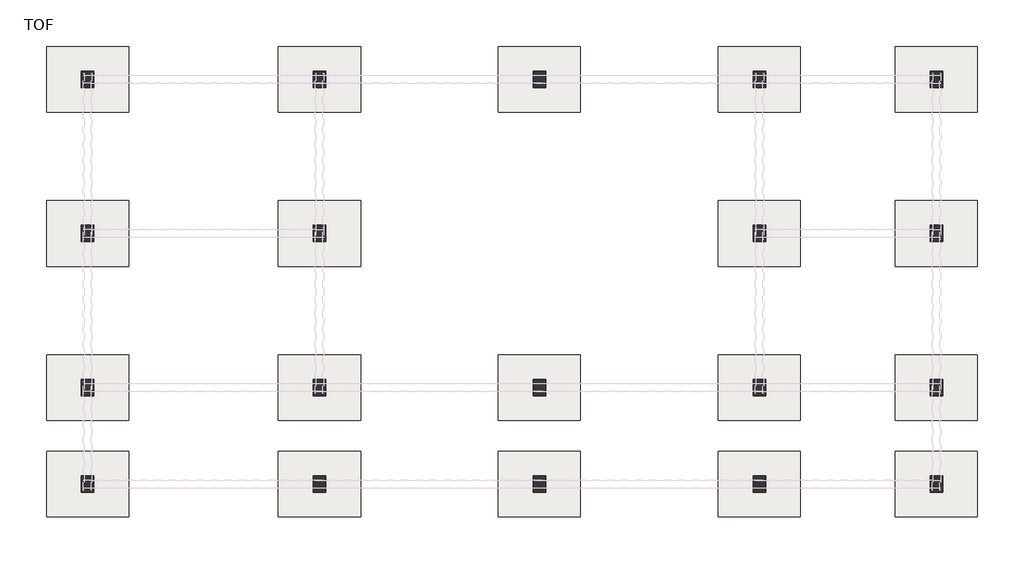
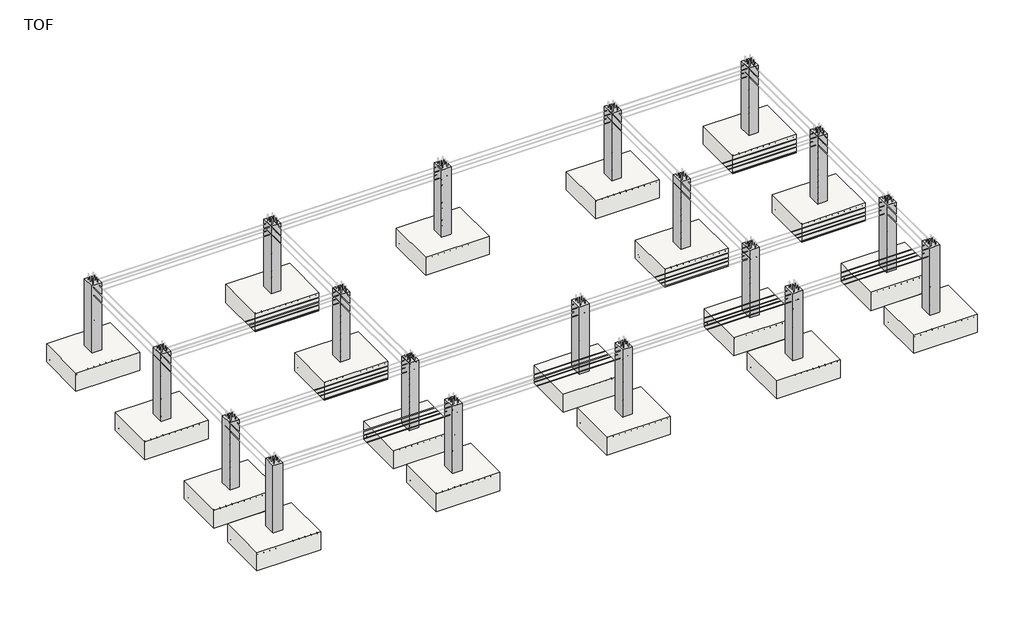
# One storey, part 1 of 10: 19 columns, 19 slabs.
"""IFC4 building model written with IfcOpenShell, lengths in millimetres."""

from ifc_helpers import new_model, si_unit, frame, origin, place, context, project, spatial, polyline, outline, extrude, transform, mapped, element, save
from components import m_footing_rectangular_1500_x_1200_x_450mm_2_af0c1bbe

model = new_model("IFC4")

# Units and contexts
model_context = context("Model", 3, world=origin())
ifc_project = project(units=[si_unit("LENGTHUNIT", "METRE", prefix="MILLI")], contexts=[model_context])

# Site, building, storey
site = spatial("IfcSite", under=ifc_project)
building = spatial("IfcBuilding", under=site)
storey = spatial("IfcBuildingStorey", under=building, Name="TOF", Elevation=-1828.8)

# Columns
placement = place(None, origin())
element("IfcColumn", 1, ObjectType="M_Concrete-Rectangular-Column : 230 x 300mm 2", at=placement, inside=storey, context=model_context, shape_type="SweptSolid", body=[
    extrude(outline(polyline([(-2504.7217857, -14944.6267376), (-2504.7217857, -15244.6267376), (-2734.7217857, -15244.6267376), (-2734.7217857, -14944.6267376), (-2504.7217857, -14944.6267376)])), frame((0.0, 0.0, -1828.8), z_axis=(0.0, 0.0, 1.0), x_axis=(1.0, 0.0, 0.0)), (0.0, 0.0, 1.0), 1678.8),
])
element("IfcColumn", 2, ObjectType="M_Concrete-Rectangular-Column : 230 x 300mm 2", at=placement, inside=storey, context=model_context, shape_type="SweptSolid", body=[
    extrude(outline(polyline([(1725.2782143, -14944.6267376), (1725.2782143, -15244.6267376), (1495.2782143, -15244.6267376), (1495.2782143, -14944.6267376), (1725.2782143, -14944.6267376)])), frame((0.0, 0.0, -1828.8), z_axis=(0.0, 0.0, 1.0), x_axis=(1.0, 0.0, 0.0)), (0.0, 0.0, 1.0), 1678.8),
])
element("IfcColumn", 3, ObjectType="M_Concrete-Rectangular-Column : 230 x 300mm 2", at=placement, inside=storey, context=model_context, shape_type="SweptSolid", body=[
    extrude(outline(polyline([(5740.2782143, -14944.6267376), (5740.2782143, -15244.6267376), (5510.2782143, -15244.6267376), (5510.2782143, -14944.6267376), (5740.2782143, -14944.6267376)])), frame((0.0, 0.0, -1828.8), z_axis=(0.0, 0.0, 1.0), x_axis=(1.0, 0.0, 0.0)), (0.0, 0.0, 1.0), 1678.8),
])
element("IfcColumn", 4, ObjectType="M_Concrete-Rectangular-Column : 230 x 300mm 2", at=placement, inside=storey, context=model_context, shape_type="SweptSolid", body=[
    extrude(outline(polyline([(9755.2782143, -14944.6267376), (9755.2782143, -15244.6267376), (9525.2782143, -15244.6267376), (9525.2782143, -14944.6267376), (9755.2782143, -14944.6267376)])), frame((0.0, 0.0, -1828.8), z_axis=(0.0, 0.0, 1.0), x_axis=(1.0, 0.0, 0.0)), (0.0, 0.0, 1.0), 1678.8),
])
element("IfcColumn", 5, ObjectType="M_Concrete-Rectangular-Column : 230 x 300mm 2", at=placement, inside=storey, context=model_context, shape_type="SweptSolid", body=[
    extrude(outline(polyline([(12985.2782143, -14944.6267376), (12985.2782143, -15244.6267376), (12755.2782143, -15244.6267376), (12755.2782143, -14944.6267376), (12985.2782143, -14944.6267376)])), frame((0.0, 0.0, -1828.8), z_axis=(0.0, 0.0, 1.0), x_axis=(1.0, 0.0, 0.0)), (0.0, 0.0, 1.0), 1678.8),
])
element("IfcColumn", 6, ObjectType="M_Concrete-Rectangular-Column : 230 x 300mm 2", at=placement, inside=storey, context=model_context, shape_type="SweptSolid", body=[
    extrude(outline(polyline([(-2504.7217857, -13179.6267376), (-2504.7217857, -13479.6267376), (-2734.7217857, -13479.6267376), (-2734.7217857, -13179.6267376), (-2504.7217857, -13179.6267376)])), frame((0.0, 0.0, -1828.8), z_axis=(0.0, 0.0, 1.0), x_axis=(1.0, 0.0, 0.0)), (0.0, 0.0, 1.0), 1678.8),
])
element("IfcColumn", 7, ObjectType="M_Concrete-Rectangular-Column : 230 x 300mm 2", at=placement, inside=storey, context=model_context, shape_type="SweptSolid", body=[
    extrude(outline(polyline([(1725.2782143, -13179.6267376), (1725.2782143, -13479.6267376), (1495.2782143, -13479.6267376), (1495.2782143, -13179.6267376), (1725.2782143, -13179.6267376)])), frame((0.0, 0.0, -1828.8), z_axis=(0.0, 0.0, 1.0), x_axis=(1.0, 0.0, 0.0)), (0.0, 0.0, 1.0), 1678.8),
])
element("IfcColumn", 8, ObjectType="M_Concrete-Rectangular-Column : 230 x 300mm 2", at=placement, inside=storey, context=model_context, shape_type="SweptSolid", body=[
    extrude(outline(polyline([(5740.2782143, -13179.6267376), (5740.2782143, -13479.6267376), (5510.2782143, -13479.6267376), (5510.2782143, -13179.6267376), (5740.2782143, -13179.6267376)])), frame((0.0, 0.0, -1828.8), z_axis=(0.0, 0.0, 1.0), x_axis=(1.0, 0.0, 0.0)), (0.0, 0.0, 1.0), 1678.8),
])
element("IfcColumn", 9, ObjectType="M_Concrete-Rectangular-Column : 230 x 300mm 2", at=placement, inside=storey, context=model_context, shape_type="SweptSolid", body=[
    extrude(outline(polyline([(9755.2782143, -13179.6267376), (9755.2782143, -13479.6267376), (9525.2782143, -13479.6267376), (9525.2782143, -13179.6267376), (9755.2782143, -13179.6267376)])), frame((0.0, 0.0, -1828.8), z_axis=(0.0, 0.0, 1.0), x_axis=(1.0, 0.0, 0.0)), (0.0, 0.0, 1.0), 1678.8),
])
element("IfcColumn", 10, ObjectType="M_Concrete-Rectangular-Column : 230 x 300mm 2", at=placement, inside=storey, context=model_context, shape_type="SweptSolid", body=[
    extrude(outline(polyline([(12985.2782143, -13179.6267376), (12985.2782143, -13479.6267376), (12755.2782143, -13479.6267376), (12755.2782143, -13179.6267376), (12985.2782143, -13179.6267376)])), frame((0.0, 0.0, -1828.8), z_axis=(0.0, 0.0, 1.0), x_axis=(1.0, 0.0, 0.0)), (0.0, 0.0, 1.0), 1678.8),
])
element("IfcColumn", 11, ObjectType="M_Concrete-Rectangular-Column : 230 x 300mm 2", at=placement, inside=storey, context=model_context, shape_type="SweptSolid", body=[
    extrude(outline(polyline([(-2504.7217857, -10364.6267376), (-2504.7217857, -10664.6267376), (-2734.7217857, -10664.6267376), (-2734.7217857, -10364.6267376), (-2504.7217857, -10364.6267376)])), frame((0.0, 0.0, -1828.8), z_axis=(0.0, 0.0, 1.0), x_axis=(1.0, 0.0, 0.0)), (0.0, 0.0, 1.0), 1678.8),
])
element("IfcColumn", 12, ObjectType="M_Concrete-Rectangular-Column : 230 x 300mm 2", at=placement, inside=storey, context=model_context, shape_type="SweptSolid", body=[
    extrude(outline(polyline([(1725.2782143, -10364.6267376), (1725.2782143, -10664.6267376), (1495.2782143, -10664.6267376), (1495.2782143, -10364.6267376), (1725.2782143, -10364.6267376)])), frame((0.0, 0.0, -1828.8), z_axis=(0.0, 0.0, 1.0), x_axis=(1.0, 0.0, 0.0)), (0.0, 0.0, 1.0), 1678.8),
])
element("IfcColumn", 13, ObjectType="M_Concrete-Rectangular-Column : 230 x 300mm 2", at=placement, inside=storey, context=model_context, shape_type="SweptSolid", body=[
    extrude(outline(polyline([(9755.2782143, -10364.6267376), (9755.2782143, -10664.6267376), (9525.2782143, -10664.6267376), (9525.2782143, -10364.6267376), (9755.2782143, -10364.6267376)])), frame((0.0, 0.0, -1828.8), z_axis=(0.0, 0.0, 1.0), x_axis=(1.0, 0.0, 0.0)), (0.0, 0.0, 1.0), 1678.8),
])
element("IfcColumn", 14, ObjectType="M_Concrete-Rectangular-Column : 230 x 300mm 2", at=placement, inside=storey, context=model_context, shape_type="SweptSolid", body=[
    extrude(outline(polyline([(12985.2782143, -10364.6267376), (12985.2782143, -10664.6267376), (12755.2782143, -10664.6267376), (12755.2782143, -10364.6267376), (12985.2782143, -10364.6267376)])), frame((0.0, 0.0, -1828.8), z_axis=(0.0, 0.0, 1.0), x_axis=(1.0, 0.0, 0.0)), (0.0, 0.0, 1.0), 1678.8),
])
element("IfcColumn", 15, ObjectType="M_Concrete-Rectangular-Column : 230 x 300mm 2", at=placement, inside=storey, context=model_context, shape_type="SweptSolid", body=[
    extrude(outline(polyline([(-2504.7217857, -7549.6267376), (-2504.7217857, -7849.6267376), (-2734.7217857, -7849.6267376), (-2734.7217857, -7549.6267376), (-2504.7217857, -7549.6267376)])), frame((0.0, 0.0, -1828.8), z_axis=(0.0, 0.0, 1.0), x_axis=(1.0, 0.0, 0.0)), (0.0, 0.0, 1.0), 1678.8),
])
element("IfcColumn", 16, ObjectType="M_Concrete-Rectangular-Column : 230 x 300mm 2", at=placement, inside=storey, context=model_context, shape_type="SweptSolid", body=[
    extrude(outline(polyline([(1725.2782143, -7549.6267376), (1725.2782143, -7849.6267376), (1495.2782143, -7849.6267376), (1495.2782143, -7549.6267376), (1725.2782143, -7549.6267376)])), frame((0.0, 0.0, -1828.8), z_axis=(0.0, 0.0, 1.0), x_axis=(1.0, 0.0, 0.0)), (0.0, 0.0, 1.0), 1678.8),
])
element("IfcColumn", 17, ObjectType="M_Concrete-Rectangular-Column : 230 x 300mm 2", at=placement, inside=storey, context=model_context, shape_type="SweptSolid", body=[
    extrude(outline(polyline([(5740.2782143, -7549.6267376), (5740.2782143, -7849.6267376), (5510.2782143, -7849.6267376), (5510.2782143, -7549.6267376), (5740.2782143, -7549.6267376)])), frame((0.0, 0.0, -1828.8), z_axis=(0.0, 0.0, 1.0), x_axis=(1.0, 0.0, 0.0)), (0.0, 0.0, 1.0), 1678.8),
])
element("IfcColumn", 18, ObjectType="M_Concrete-Rectangular-Column : 230 x 300mm 2", at=placement, inside=storey, context=model_context, shape_type="SweptSolid", body=[
    extrude(outline(polyline([(9755.2782143, -7549.6267376), (9755.2782143, -7849.6267376), (9525.2782143, -7849.6267376), (9525.2782143, -7549.6267376), (9755.2782143, -7549.6267376)])), frame((0.0, 0.0, -1828.8), z_axis=(0.0, 0.0, 1.0), x_axis=(1.0, 0.0, 0.0)), (0.0, 0.0, 1.0), 1678.8),
])
element("IfcColumn", 19, ObjectType="M_Concrete-Rectangular-Column : 230 x 300mm 2", at=placement, inside=storey, context=model_context, shape_type="SweptSolid", body=[
    extrude(outline(polyline([(12985.2782143, -7549.6267376), (12985.2782143, -7849.6267376), (12755.2782143, -7849.6267376), (12755.2782143, -7549.6267376), (12985.2782143, -7549.6267376)])), frame((0.0, 0.0, -1828.8), z_axis=(0.0, 0.0, 1.0), x_axis=(1.0, 0.0, 0.0)), (0.0, 0.0, 1.0), 1678.8),
])

# Slabs
m_footing_rectangular_1500_x_1200_x_450mm_2_shape = m_footing_rectangular_1500_x_1200_x_450mm_2_af0c1bbe(model_context)
element("IfcSlab", 20, ObjectType="M_Footing-Rectangular : 1500 x 1200 x 450mm 2", at=placement, inside=storey, context=model_context, shape_type="MappedRepresentation", body=[
    mapped(m_footing_rectangular_1500_x_1200_x_450mm_2_shape, transform((-2619.7217857, -15094.6267376, -1828.8), x_axis=(0.0, 1.0, 0.0), y_axis=(-1.0, 0.0, 0.0), z_axis=(0.0, 0.0, 1.0))),
])
element("IfcSlab", 21, ObjectType="M_Footing-Rectangular : 1500 x 1200 x 450mm 2", at=placement, inside=storey, context=model_context, shape_type="MappedRepresentation", body=[
    mapped(m_footing_rectangular_1500_x_1200_x_450mm_2_shape, transform((1610.2782143, -15094.6267376, -1828.8), x_axis=(0.0, 1.0, 0.0), y_axis=(-1.0, 0.0, 0.0), z_axis=(0.0, 0.0, 1.0))),
])
element("IfcSlab", 22, ObjectType="M_Footing-Rectangular : 1500 x 1200 x 450mm 2", at=placement, inside=storey, context=model_context, shape_type="MappedRepresentation", body=[
    mapped(m_footing_rectangular_1500_x_1200_x_450mm_2_shape, transform((5625.2782143, -15094.6267376, -1828.8), x_axis=(0.0, 1.0, 0.0), y_axis=(-1.0, 0.0, 0.0), z_axis=(0.0, 0.0, 1.0))),
])
element("IfcSlab", 23, ObjectType="M_Footing-Rectangular : 1500 x 1200 x 450mm 2", at=placement, inside=storey, context=model_context, shape_type="MappedRepresentation", body=[
    mapped(m_footing_rectangular_1500_x_1200_x_450mm_2_shape, transform((9640.2782143, -15094.6267376, -1828.8), x_axis=(0.0, 1.0, 0.0), y_axis=(-1.0, 0.0, 0.0), z_axis=(0.0, 0.0, 1.0))),
])
element("IfcSlab", 24, ObjectType="M_Footing-Rectangular : 1500 x 1200 x 450mm 2", at=placement, inside=storey, context=model_context, shape_type="MappedRepresentation", body=[
    mapped(m_footing_rectangular_1500_x_1200_x_450mm_2_shape, transform((12870.2782143, -15094.6267376, -1828.8), x_axis=(0.0, 1.0, 0.0), y_axis=(-1.0, 0.0, 0.0), z_axis=(0.0, 0.0, 1.0))),
])
element("IfcSlab", 25, ObjectType="M_Footing-Rectangular : 1500 x 1200 x 450mm 2", at=placement, inside=storey, context=model_context, shape_type="MappedRepresentation", body=[
    mapped(m_footing_rectangular_1500_x_1200_x_450mm_2_shape, transform((-2619.7217857, -13329.6267376, -1828.8), x_axis=(0.0, 1.0, 0.0), y_axis=(-1.0, 0.0, 0.0), z_axis=(0.0, 0.0, 1.0))),
])
element("IfcSlab", 26, ObjectType="M_Footing-Rectangular : 1500 x 1200 x 450mm 2", at=placement, inside=storey, context=model_context, shape_type="MappedRepresentation", body=[
    mapped(m_footing_rectangular_1500_x_1200_x_450mm_2_shape, transform((1610.2782143, -13329.6267376, -1828.8), x_axis=(0.0, 1.0, 0.0), y_axis=(-1.0, 0.0, 0.0), z_axis=(0.0, 0.0, 1.0))),
])
element("IfcSlab", 27, ObjectType="M_Footing-Rectangular : 1500 x 1200 x 450mm 2", at=placement, inside=storey, context=model_context, shape_type="MappedRepresentation", body=[
    mapped(m_footing_rectangular_1500_x_1200_x_450mm_2_shape, transform((5625.2782143, -13329.6267376, -1828.8), x_axis=(0.0, 1.0, 0.0), y_axis=(-1.0, 0.0, 0.0), z_axis=(0.0, 0.0, 1.0))),
])
element("IfcSlab", 28, ObjectType="M_Footing-Rectangular : 1500 x 1200 x 450mm 2", at=placement, inside=storey, context=model_context, shape_type="MappedRepresentation", body=[
    mapped(m_footing_rectangular_1500_x_1200_x_450mm_2_shape, transform((9640.2782143, -13329.6267376, -1828.8), x_axis=(0.0, 1.0, 0.0), y_axis=(-1.0, 0.0, 0.0), z_axis=(0.0, 0.0, 1.0))),
])
element("IfcSlab", 29, ObjectType="M_Footing-Rectangular : 1500 x 1200 x 450mm 2", at=placement, inside=storey, context=model_context, shape_type="MappedRepresentation", body=[
    mapped(m_footing_rectangular_1500_x_1200_x_450mm_2_shape, transform((12870.2782143, -13329.6267376, -1828.8), x_axis=(0.0, 1.0, 0.0), y_axis=(-1.0, 0.0, 0.0), z_axis=(0.0, 0.0, 1.0))),
])
element("IfcSlab", 30, ObjectType="M_Footing-Rectangular : 1500 x 1200 x 450mm 2", at=placement, inside=storey, context=model_context, shape_type="MappedRepresentation", body=[
    mapped(m_footing_rectangular_1500_x_1200_x_450mm_2_shape, transform((-2619.7217857, -10514.6267376, -1828.8), x_axis=(0.0, 1.0, 0.0), y_axis=(-1.0, 0.0, 0.0), z_axis=(0.0, 0.0, 1.0))),
])
element("IfcSlab", 31, ObjectType="M_Footing-Rectangular : 1500 x 1200 x 450mm 2", at=placement, inside=storey, context=model_context, shape_type="MappedRepresentation", body=[
    mapped(m_footing_rectangular_1500_x_1200_x_450mm_2_shape, transform((1610.2782143, -10514.6267376, -1828.8), x_axis=(0.0, 1.0, 0.0), y_axis=(-1.0, 0.0, 0.0), z_axis=(0.0, 0.0, 1.0))),
])
element("IfcSlab", 32, ObjectType="M_Footing-Rectangular : 1500 x 1200 x 450mm 2", at=placement, inside=storey, context=model_context, shape_type="MappedRepresentation", body=[
    mapped(m_footing_rectangular_1500_x_1200_x_450mm_2_shape, transform((9640.2782143, -10514.6267376, -1828.8), x_axis=(0.0, 1.0, 0.0), y_axis=(-1.0, 0.0, 0.0), z_axis=(0.0, 0.0, 1.0))),
])
element("IfcSlab", 33, ObjectType="M_Footing-Rectangular : 1500 x 1200 x 450mm 2", at=placement, inside=storey, context=model_context, shape_type="MappedRepresentation", body=[
    mapped(m_footing_rectangular_1500_x_1200_x_450mm_2_shape, transform((12870.2782143, -10514.6267376, -1828.8), x_axis=(0.0, 1.0, 0.0), y_axis=(-1.0, 0.0, 0.0), z_axis=(0.0, 0.0, 1.0))),
])
element("IfcSlab", 34, ObjectType="M_Footing-Rectangular : 1500 x 1200 x 450mm 2", at=placement, inside=storey, context=model_context, shape_type="MappedRepresentation", body=[
    mapped(m_footing_rectangular_1500_x_1200_x_450mm_2_shape, transform((-2619.7217857, -7699.6267376, -1828.8), x_axis=(0.0, 1.0, 0.0), y_axis=(-1.0, 0.0, 0.0), z_axis=(0.0, 0.0, 1.0))),
])
element("IfcSlab", 35, ObjectType="M_Footing-Rectangular : 1500 x 1200 x 450mm 2", at=placement, inside=storey, context=model_context, shape_type="MappedRepresentation", body=[
    mapped(m_footing_rectangular_1500_x_1200_x_450mm_2_shape, transform((1610.2782143, -7699.6267376, -1828.8), x_axis=(0.0, 1.0, 0.0), y_axis=(-1.0, 0.0, 0.0), z_axis=(0.0, 0.0, 1.0))),
])
element("IfcSlab", 36, ObjectType="M_Footing-Rectangular : 1500 x 1200 x 450mm 2", at=placement, inside=storey, context=model_context, shape_type="MappedRepresentation", body=[
    mapped(m_footing_rectangular_1500_x_1200_x_450mm_2_shape, transform((5625.2782143, -7699.6267376, -1828.8), x_axis=(0.0, 1.0, 0.0), y_axis=(-1.0, 0.0, 0.0), z_axis=(0.0, 0.0, 1.0))),
])
element("IfcSlab", 37, ObjectType="M_Footing-Rectangular : 1500 x 1200 x 450mm 2", at=placement, inside=storey, context=model_context, shape_type="MappedRepresentation", body=[
    mapped(m_footing_rectangular_1500_x_1200_x_450mm_2_shape, transform((9640.2782143, -7699.6267376, -1828.8), x_axis=(0.0, 1.0, 0.0), y_axis=(-1.0, 0.0, 0.0), z_axis=(0.0, 0.0, 1.0))),
])
element("IfcSlab", 38, ObjectType="M_Footing-Rectangular : 1500 x 1200 x 450mm 2", at=placement, inside=storey, context=model_context, shape_type="MappedRepresentation", body=[
    mapped(m_footing_rectangular_1500_x_1200_x_450mm_2_shape, transform((12870.2782143, -7699.6267376, -1828.8), x_axis=(0.0, 1.0, 0.0), y_axis=(-1.0, 0.0, 0.0), z_axis=(0.0, 0.0, 1.0))),
])

save(model, "model.ifc")

# Revit data of these elements
# Grids (mm)
#   "1": line (15899.329, -15094.627) -> (-5005.909, -15094.627)
#   "2": line (15899.329, -13329.627) -> (-5005.909, -13329.627)
#   "3": line (15899.329, -10514.627) -> (-5005.909, -10514.627)
#   "4": line (15899.329, -7699.627) -> (-5005.909, -7699.627)
#   "A": line (-2619.722, -16952.66) -> (-2619.722, -5620.21)
#   "B": line (1610.278, -16952.66) -> (1610.278, -5620.21)
#   "C": line (5625.278, -16952.66) -> (5625.278, -5620.21)
#   "D": line (9640.278, -16952.66) -> (9640.278, -5620.21)
#   "E": line (12870.278, -16952.66) -> (12870.278, -5620.21)
# Type "M_Concrete-Rectangular-Column : 230 x 300mm 2"
#   b = 0' - 9.05512"
#   h = 0' - 11.81102"
#   Structural Material [instance default] = Concrete, Cast-in-Place gray
# Type "M_Footing-Rectangular : 1500 x 1200 x 450mm 2"
#   Width = 3' - 11.24409"
#   Length = 4' - 11.05512"
#   Foundation Thickness = 1' - 5.71654"
#   Structural Material [instance default] = Concrete, Cast-in-Place gray
#   Assembly Code = ""
# Elements 1, 2, 3, 4, 5, 6, 7, 8, 9, 10, 11, 12, 13, 14, 15, 16, 17, 18, 19 (IfcColumn, "M_Concrete-Rectangular-Column : 230 x 300mm 2")
#   Structural Material = Concrete, Cast-in-Place gray
#   Phase Created = New Construction
#   Materials on its faces: "Concrete, Cast-in-Place gray"
# Elements 20, 21, 22, 23, 24, 25, 26, 27, 28, 29, 30, 31, 32, 33, 34, 35, 36, 37, 38 (IfcSlab, "M_Footing-Rectangular : 1500 x 1200 x 450mm 2")
#   Structural Material = Concrete, Cast-in-Place gray
#   Phase Created = New Construction
#   Materials on its faces: "Concrete, Cast-in-Place gray"
# Materials
#   "Concrete, Cast-in-Place gray": class "Concrete", colour RGB 192 192 192, transparency 0, Description = "Cast-in-place concrete", Cost = 0
